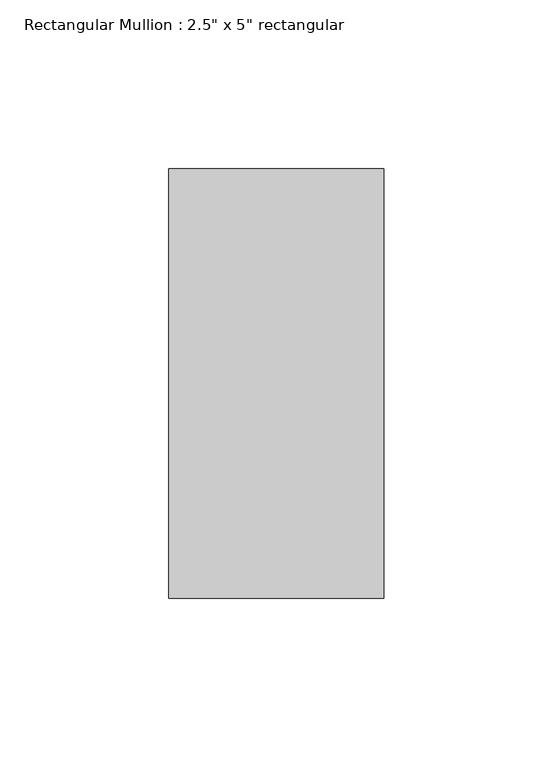
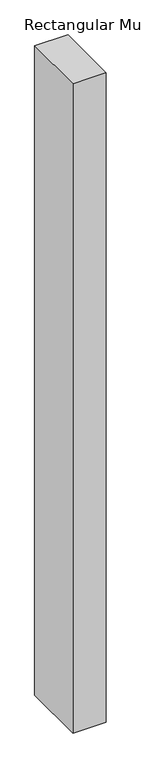
"""IFC4 building model written with IfcOpenShell, lengths in millimetres: member geometry."""

from ifc_helpers import new_model, si_unit, frame, origin, place, context, project, spatial, polyline, outline, extrude, source, transform, mapped, element, save


def member_af85eb51(model_context):
    return source(origin(), model_context, "Body", "SweptSolid", [
        extrude(outline(polyline([(0.0, 63.5), (0.0, -63.5), (-63.5, -63.5), (-63.5, 63.5), (0.0, 63.5)])), frame((0.0, 0.0, -1315.1739179), z_axis=(0.0, 0.0, 1.0), x_axis=(1.0, 0.0, 0.0)), (0.0, 0.0, 1.0), 1315.1739179),
    ])


if __name__ == "__main__":
    model = new_model("IFC4")
    model_context = context("Model", 3, world=origin())
    ifc_project = project(units=[si_unit("LENGTHUNIT", "METRE", prefix="MILLI")], contexts=[model_context])
    site = spatial("IfcSite", under=ifc_project)
    building = spatial("IfcBuilding", under=site)
    placement = place(None, origin())
    member_shape = member_af85eb51(model_context)
    element("IfcMember", 1, ObjectType="Rectangular Mullion : 2.5\" x 5\" rectangular", at=placement, inside=building, context=model_context, shape_type="MappedRepresentation", body=[
        mapped(member_shape, transform((0.0, 0.0, 0.0), x_axis=(1.0, 0.0, 0.0), y_axis=(0.0, 1.0, 0.0), z_axis=(0.0, 0.0, 1.0))),
    ])
    save(model, "model.ifc")

# Revit data of these elements
# Type "Rectangular Mullion : 2.5\" x 5\" rectangular"
#   built-in parameter 1007304 = 0.416667 (stored number, unit not read)
#   built-in parameter 1007301 = 0.104167 (stored number, unit not read)
#   built-in parameter 1007300 = 0.104167 (stored number, unit not read)
# Element 1 (IfcMember, "Rectangular Mullion : 2.5\" x 5\" rectangular")
#   Materials on its faces: "Aluminum"
# Materials
#   "Aluminum": class "Metal", colour RGB 247 247 247, transparency 0, Description = "Aluminum 6061", Cost = 0
